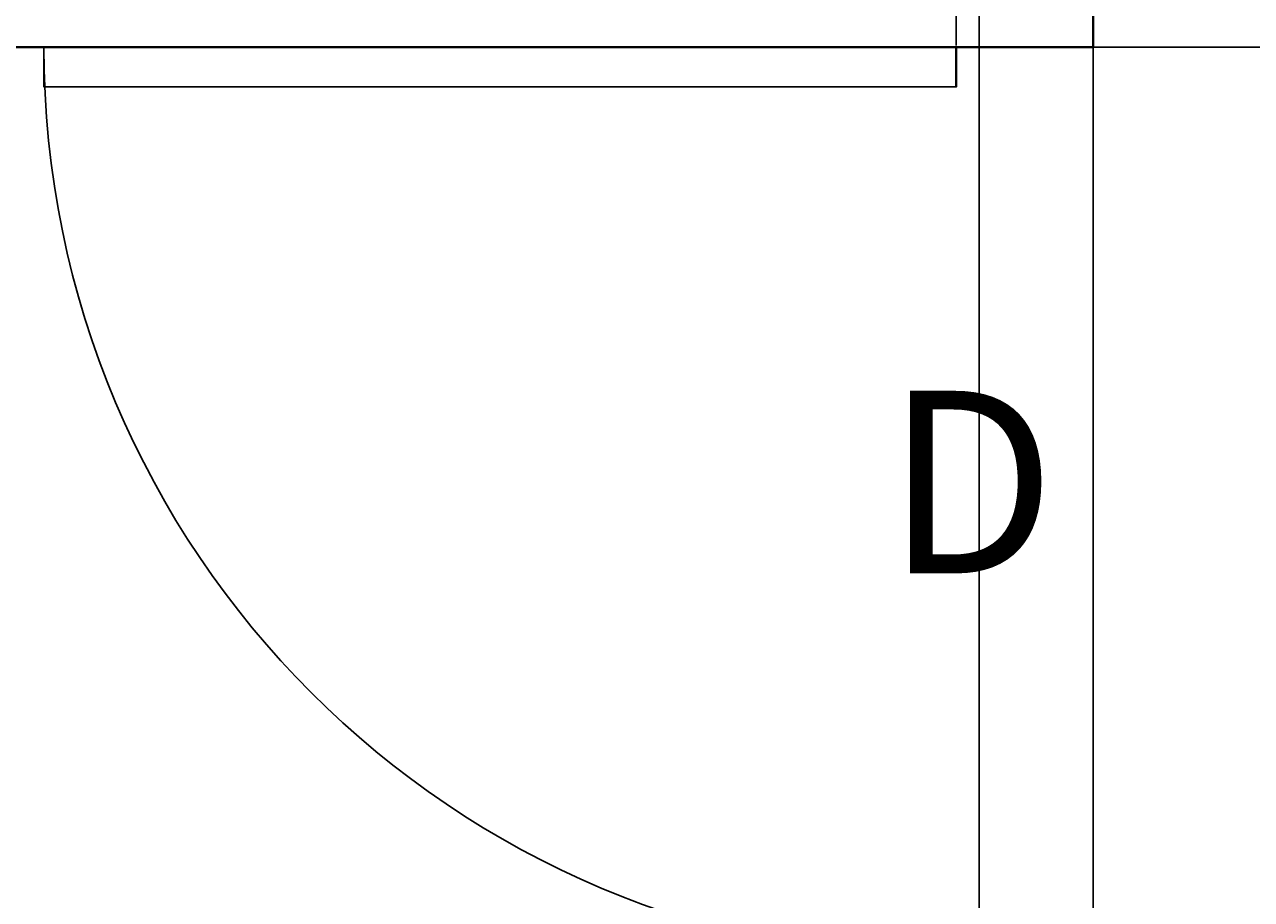
# Model space of a CAD drawing. Units: inches. Extents: x -301 to 715, y -607 to 364.
# Tile 85 of 141: x -92 to -39, y 28 to 67. Entities that reach past the tile are written whole.
import ezdxf

# ---------------------------------------------------------------- set-up
doc = ezdxf.new("R2010")
doc.units = ezdxf.units.IN
doc.header["$MEASUREMENT"] = 0
for name, color, linetype, lineweight in [('A-ANNO-DIMS', 2, 'Continuous', 18), ('A-ANNO-TEXT', 4, 'Continuous', 18), ('A-DOOR', 4, 'Continuous', 25), ('A-WALL', 3, 'Continuous', 40)]:
    doc.layers.add(name, color=color, linetype=linetype, lineweight=lineweight)
doc.styles.get("Standard").update_dxf_attribs({"font": 'arial.ttf'})
doc.dimstyles.get("Standard").update_dxf_attribs({"dimtxt": 0.18, "dimasz": 0.18, "dimexe": 0.18, "dimexo": 0.0625, "dimgap": 0.09, "dimtad": 0, "dimtih": 1, "dimtoh": 1, "dimdec": 1, "dimzin": 0, "dimdsep": 46, "dimlunit": 4, "dimtxsty": 'Standard', "dimcen": 0.09, "dimclrd": 3, "dimclre": 4, "dimclrt": 6, "dimadec": 0, "dimazin": 0, "dimtfac": 1, "dimtdec": 1, "dimtofl": 0, "dimtmove": 0, "dimatfit": 3, "dimfxl": 1, "dimtfill": 2, "dimtfillclr": 51, "dimtolj": 1, "dimtzin": 0, "dimarcsym": 0})

# ---------------------------------------------------------------- blocks, each defined once
blk = doc.blocks.new('*U5')
for p, q in [((0, 0), (0, -6)), ((-40, 0), (-40, -6))]:
    blk.add_line(p, q)
blk.add_lwpolyline([(0, 0), (0, 40), (-1.75, 40), (-1.75, 0)], close=True)
blk.add_arc((0, 0), 40, 90, 180)
blk = doc.blocks.new('*D149')
at = {"layer": 'A-ANNO-DIMS', "color": 4, "lineweight": -2, "transparency": 16777216}
for p, q in [((-51.541, 65.682), (233.659, 65.682)), ((-51.541, 25.682), (233.659, 25.682))]:
    blk.add_line(p, q, dxfattribs=at)
at = {"layer": 'A-ANNO-DIMS', "color": 3, "lineweight": -2, "transparency": 16777216}
for p, q in [((233.479, 65.502), (233.479, 45.864)), ((233.479, 25.862), (233.479, 45.5))]:
    blk.add_line(p, q, dxfattribs=at)
at = {"layer": 'A-ANNO-DIMS', "color": 3, "transparency": 16777216}
for points in [[(233.449, 65.502), (233.509, 65.502), (233.479, 65.682)], [(233.449, 25.862), (233.509, 25.862), (233.479, 25.682)]]:
    blk.add_solid(points, dxfattribs=at)
at = {"layer": 'Defpoints', "color": 0, "transparency": 16777216}
for p in [(-51.603, 65.682), (-51.603, 25.682), (233.479, 25.682)]:
    blk.add_point(p, dxfattribs=at)
at = {"layer": 'A-ANNO-DIMS', "color": 6, "transparency": 16777216, "insert": (233.479, 45.682), "char_height": 0.18, "attachment_point": 5, "bg_fill": 1, "box_fill_scale": 1.25, "bg_fill_color": 51, "bg_fill_transparency": 0}
blk.add_mtext('\\A1;3\'-4"', dxfattribs=at)
blk = doc.blocks.new('*D150')
at = {"layer": 'A-ANNO-DIMS', "color": 4, "lineweight": -2, "transparency": 16777216}
for p, q in [((-51.603, 65.745), (-51.603, 359.612)), ((-45.603, 65.745), (-45.603, 359.612))]:
    blk.add_line(p, q, dxfattribs=at)
at = {"layer": 'A-ANNO-DIMS', "color": 3, "lineweight": -2, "transparency": 16777216}
for p, q in [((-51.423, 359.432), (-48.933, 359.432)), ((-45.783, 359.432), (-48.274, 359.432))]:
    blk.add_line(p, q, dxfattribs=at)
at = {"layer": 'A-ANNO-DIMS', "color": 3, "transparency": 16777216}
for points in [[(-51.423, 359.462), (-51.423, 359.402), (-51.603, 359.432)], [(-45.783, 359.462), (-45.783, 359.402), (-45.603, 359.432)]]:
    blk.add_solid(points, dxfattribs=at)
at = {"layer": 'Defpoints', "color": 0, "transparency": 16777216}
for p in [(-51.603, 359.432), (-51.603, 65.682), (-45.603, 65.682)]:
    blk.add_point(p, dxfattribs=at)
at = {"layer": 'A-ANNO-DIMS', "color": 6, "transparency": 16777216, "insert": (-48.603, 359.432), "char_height": 0.18, "attachment_point": 5, "bg_fill": 1, "box_fill_scale": 1.25, "bg_fill_color": 51, "bg_fill_transparency": 0}
blk.add_mtext('\\A1;0\'-6"', dxfattribs=at)
blk = doc.blocks.new('*D151')
at = {"layer": 'A-ANNO-DIMS', "color": 4, "lineweight": -2, "transparency": 16777216}
for p, q in [((-204.603, -223.755), (-204.603, 359.612)), ((-45.603, -214.755), (-45.603, 359.612))]:
    blk.add_line(p, q, dxfattribs=at)
at = {"layer": 'A-ANNO-DIMS', "color": 3, "lineweight": -2, "transparency": 16777216}
for p, q in [((-204.423, 359.432), (-125.494, 359.432)), ((-45.783, 359.432), (-124.713, 359.432))]:
    blk.add_line(p, q, dxfattribs=at)
at = {"layer": 'A-ANNO-DIMS', "color": 3, "transparency": 16777216}
for points in [[(-204.423, 359.462), (-204.423, 359.402), (-204.603, 359.432)], [(-45.783, 359.462), (-45.783, 359.402), (-45.603, 359.432)]]:
    blk.add_solid(points, dxfattribs=at)
at = {"layer": 'Defpoints', "color": 0, "transparency": 16777216}
for p in [(-45.603, 359.432), (-45.603, -214.818), (-204.603, -223.818)]:
    blk.add_point(p, dxfattribs=at)
at = {"layer": 'A-ANNO-DIMS', "color": 6, "transparency": 16777216, "insert": (-125.103, 359.432), "char_height": 0.18, "attachment_point": 5, "bg_fill": 1, "box_fill_scale": 1.25, "bg_fill_color": 51, "bg_fill_transparency": 0}
blk.add_mtext('\\A1;13\'-3"', dxfattribs=at)
blk = doc.blocks.new('*D158')
at = {"layer": 'A-ANNO-DIMS', "color": 4, "lineweight": -2, "transparency": 16777216}
for p, q in [((-122.603, 221.62), (-122.603, -296.865)), ((-50.603, 221.62), (-50.603, -296.865))]:
    blk.add_line(p, q, dxfattribs=at)
at = {"layer": 'A-ANNO-DIMS', "color": 3, "lineweight": -2, "transparency": 16777216}
for p, q in [((-122.423, -296.685), (-86.933, -296.685)), ((-50.783, -296.685), (-86.274, -296.685))]:
    blk.add_line(p, q, dxfattribs=at)
at = {"layer": 'A-ANNO-DIMS', "color": 3, "transparency": 16777216}
for points in [[(-122.423, -296.655), (-122.423, -296.715), (-122.603, -296.685)], [(-50.783, -296.655), (-50.783, -296.715), (-50.603, -296.685)]]:
    blk.add_solid(points, dxfattribs=at)
at = {"layer": 'Defpoints', "color": 0, "transparency": 16777216}
for p in [(-122.603, 221.682), (-50.603, 221.682), (-50.603, -296.685)]:
    blk.add_point(p, dxfattribs=at)
at = {"layer": 'A-ANNO-DIMS', "color": 6, "transparency": 16777216, "insert": (-86.603, -296.685), "char_height": 0.18, "attachment_point": 5, "bg_fill": 1, "box_fill_scale": 1.25, "bg_fill_color": 51, "bg_fill_transparency": 0}
blk.add_mtext('\\A1;6\'-0"', dxfattribs=at)

msp = doc.modelspace()

# ---------------------------------------------------------------- linework, layer by layer
at = {"layer": 'A-WALL'}
for p, q in [((-45.603, 65.682), (-45.603, 71.682)), ((-45.603, 65.682), (-195.603, 65.682)), ((-51.603, 63.932), (-51.603, 65.682))]:
    msp.add_line(p, q, dxfattribs=at)

# ---------------------------------------------------------------- block references
at = {"layer": 'A-DOOR', "rotation": 90}
msp.add_blockref('*U5', (-51.603, 65.682), dxfattribs=at)

# ---------------------------------------------------------------- texts
at = {"layer": 'A-ANNO-TEXT'}
msp.add_text('D', height=8, dxfattribs=at).set_placement((-54.736, 42.617))

# ---------------------------------------------------------------- dimensions: what is measured, and where the dimension line sits
at = {"layer": 'A-ANNO-DIMS'}
for base, p1, p2, picture, middle in [((-45.603, 359.432), (-204.603, -223.818), (-45.603, -214.818), '*D151', (-125.103, 359.432)), ((-51.603, 359.432), (-45.603, 65.682), (-51.603, 65.682), '*D150', (-48.603, 359.432)), ((-50.603, -296.685), (-122.603, 221.682), (-50.603, 221.682), '*D158', (-86.603, -296.685))]:
    dim = msp.add_linear_dim(base=base, p1=p1, p2=p2, dimstyle='Standard', override={"dimdec": 1, "dimlfac": 1, "dimrnd": 0, "dimzin": 1, "dimdsep": 46, "dimlunit": 4, "dimfrac": 2}, dxfattribs=at)
    dim.commit()
    dim.dimension.update_dxf_attribs({"geometry": picture, "text_midpoint": middle})
dim = msp.add_linear_dim(base=(233.479, 25.682), p1=(-51.603, 65.682), p2=(-51.603, 25.682), angle=90, dimstyle='Standard', override={"dimdec": 1, "dimlfac": 1, "dimrnd": 0, "dimzin": 1, "dimdsep": 46, "dimlunit": 4, "dimfrac": 2}, dxfattribs=at)
dim.commit()
dim.dimension.update_dxf_attribs({"geometry": '*D149', "text_midpoint": (233.479, 45.682)})

doc.saveas('drawing.dxf')
